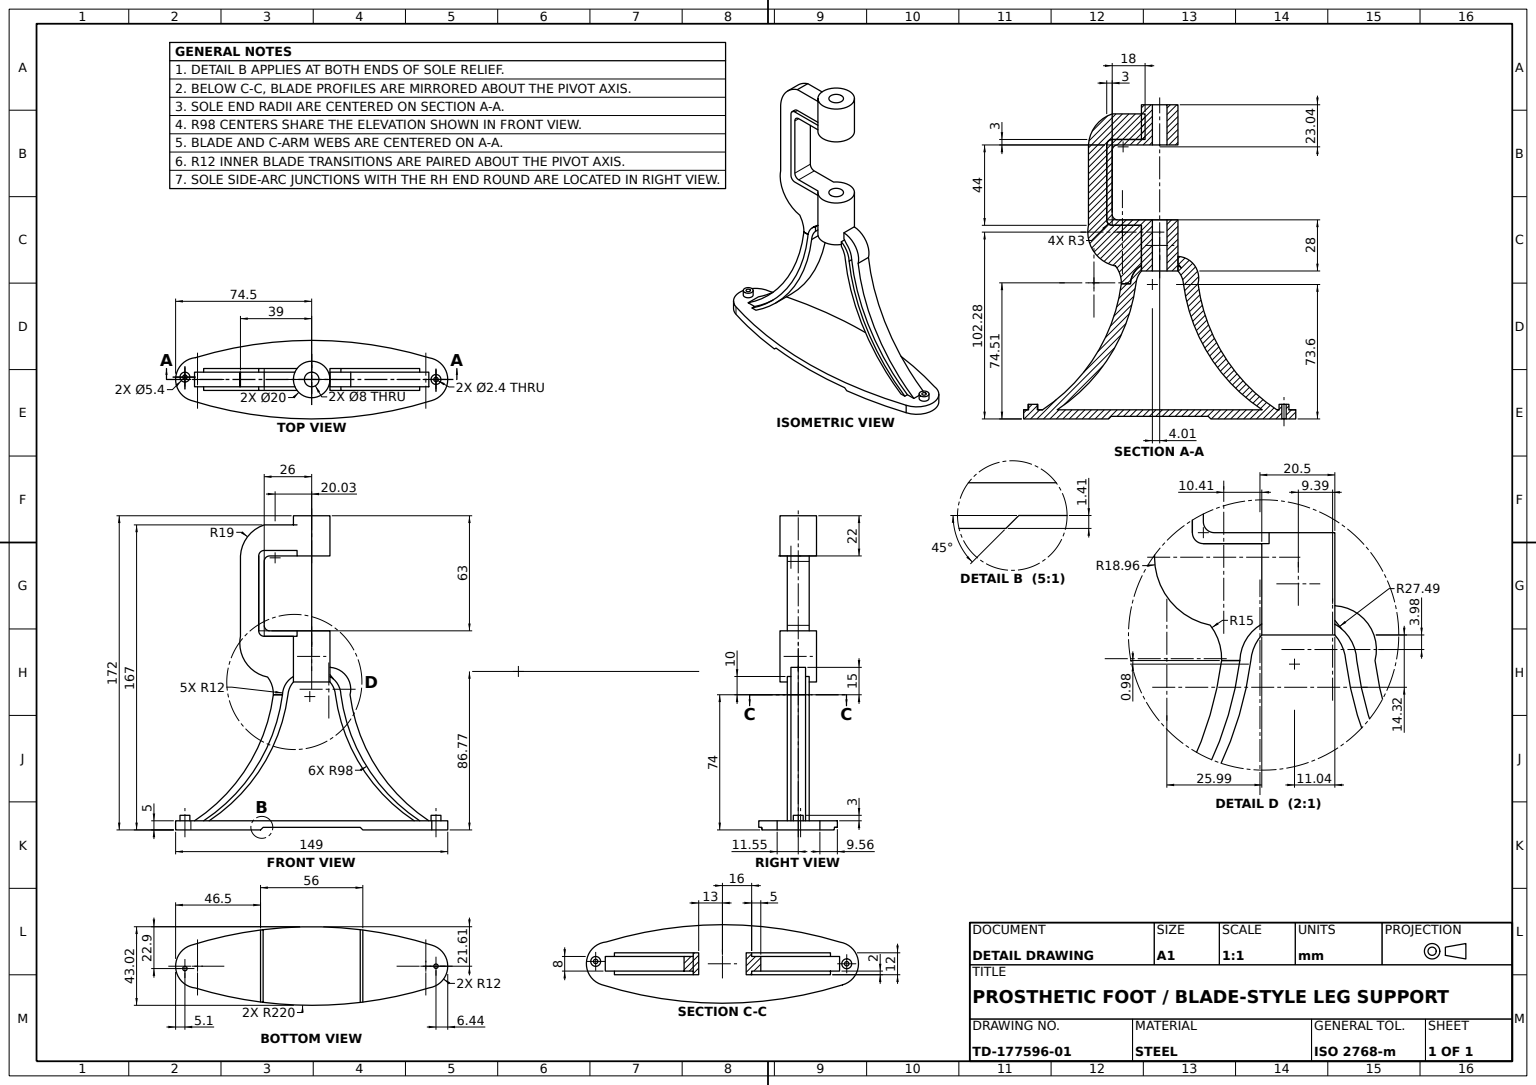
from build123d import *

# Parameters (mm, degrees)
BASE_PLATE_DEPTH             = 5
UPPER_PIVOT_BOSS_SKETCH_R    = 10
UPPER_PIVOT_BOSS_DEPTH       = 22
LOWER_PIVOT_BOSS_SKETCH_R    = 10
LOWER_PIVOT_BOSS_DEPTH       = 28
SUPPORT_LEGS_DEPTH           = 6
C_ARM_DEPTH                  = 6
LEG_RIBS_DEPTH               = 4
C_ARM_RIB_DEPTH              = 4
PIVOT_BORE_SKETCH_R          = 4
PIVOT_BORE_DEPTH             = 128
BASE_SCREW_BOSSES_SKETCH_R   = 2.697739099
BASE_SCREW_BOSSES_SKETCH_R_2 = 2.7
BASE_SCREW_BOSSES_DEPTH      = 3
BASE_SCREW_HOLES_SKETCH_R    = 1.2
BASE_SCREW_HOLES_DEPTH       = 33
PROFILE_TRIM_CUT_DEPTH       = 59


with BuildPart() as part:
    # Base Plate Sketch → Base Plate (new body)
    with BuildSketch(Plane(origin=(0, 0, 0), x_dir=(1, 0, 0), z_dir=(0, 1, 0))):
        with BuildLine():
            ThreePointArc((64.36610424, 11.854014297), (0.380988732, 21.413349806), (-63.618068043, 11.947799959))
            ThreePointArc((-63.618068043, 11.947799959), (-74.430459123, 1.290017486), (-66.146151353, -11.432654124))
            ThreePointArc((-66.146151353, -11.432654124), (-66.105249037, -11.445618349), (-66.064300627, -11.458436239))
            ThreePointArc((-66.064300627, -11.458436239), (-0.16489578, -21.609157542), (65.7488293, -11.551844363))
            ThreePointArc((65.7488293, -11.551844363), (74.479114791, 0.707678469), (64.36610424, 11.854014297))
        make_face()
    extrude(amount=BASE_PLATE_DEPTH)

    # Support Legs Sketch → Support Legs (add, symmetric)
    with BuildSketch(Plane.XY):
        with BuildLine():
            Line((-56.146151353, 5), (-59.146151353, 5))
            ThreePointArc((-59.146151353, 5), (-30.072320043, 34.809728437), (-16, 74))
            ThreePointArc((-16, 74), (-14.296453431, 79.777872059), (-10, 84))
            Line((-10, 84), (-10, 81))
            ThreePointArc((-10, 81), (-12.070047611, 77.744306119), (-13, 74))
            ThreePointArc((-13, 74), (-27.072320043, 34.809728437), (-56.146151353, 5))
        make_face()
        with BuildLine():
            Line((56.146151353, 5), (59.146151353, 5))
            ThreePointArc((59.146151353, 5), (30.072320043, 34.809728437), (16, 74))
            ThreePointArc((16, 74), (14.296453431, 79.777872059), (10, 84))
            Line((10, 84), (10, 81))
            ThreePointArc((10, 81), (12.070047611, 77.744306119), (13, 74))
            ThreePointArc((13, 74), (27.072320043, 34.809728437), (56.146151353, 5))
        make_face()
    extrude(amount=SUPPORT_LEGS_DEPTH, both=True)

    # Leg Ribs Sketch → Leg Ribs (add, symmetric)
    with BuildSketch(Plane.XY):
        with BuildLine():
            ThreePointArc((-16, 74), (-30.072320043, 34.809728437), (-59.146151353, 5))
            Line((-59.146151353, 5), (-64.146151353, 5))
            ThreePointArc((-64.146151353, 5), (-35.072320043, 34.809728437), (-21, 74))
            Line((-21, 74), (-16, 74))
        make_face()
        with BuildLine():
            ThreePointArc((16, 74), (30.072320043, 34.809728437), (59.146151353, 5))
            Line((59.146151353, 5), (64.146151353, 5))
            ThreePointArc((64.146151353, 5), (35.072320043, 34.809728437), (21, 74))
            ThreePointArc((21, 74), (19.061991309, 84.11212696), (10, 89))
            Line((10, 89), (10, 85))
            ThreePointArc((10, 85), (13.635056418, 79.84639441), (16, 74))
        make_face()
    extrude(amount=LEG_RIBS_DEPTH, both=True)

    # Base Screw Bosses Sketch → Base Screw Bosses (add)
    with BuildSketch(Plane(origin=(0, 5, 0), x_dir=(1, 0, 0), z_dir=(0, 1, 0))):
        with Locations(Location((68.059525022, 0, 0), (0, 0, 270))):
            Circle(BASE_SCREW_BOSSES_SKETCH_R)
        with Locations(Location((-69.403797915, 1.290017486, 0), (0, 0, 270))):
            Circle(BASE_SCREW_BOSSES_SKETCH_R_2)
    extrude(amount=BASE_SCREW_BOSSES_DEPTH)

    # Base Screw Holes Sketch → Base Screw Holes (cut)
    with BuildSketch(Plane(origin=(0, 8, 0), x_dir=(1, 0, 0), z_dir=(0, 1, 0))):
        with Locations(Location((68.059525022, 0, 0), (0, 0, 270))):
            Circle(BASE_SCREW_HOLES_SKETCH_R)
        with Locations(Location((-69.403797915, 1.290017486, 0), (0, 0, 270))):
            Circle(BASE_SCREW_HOLES_SKETCH_R)
    extrude(amount=-BASE_SCREW_HOLES_DEPTH, mode=Mode.SUBTRACT)

    # Profile Trim Sketch → Profile Trim Cut (cut)
    with BuildSketch(Plane.XY.offset(22)):
        Polygon((0, 0), (28, 0), (26.585786438, 1.414213562), (-26.585786438, 1.414213562), (-28, 0), align=None)
    extrude(amount=-PROFILE_TRIM_CUT_DEPTH, mode=Mode.SUBTRACT)


with BuildPart() as body_2:
    # Upper Pivot Boss Sketch → Upper Pivot Boss (new body)
    with BuildSketch(Plane(origin=(0, 172, 0), x_dir=(1, 0, 0), z_dir=(0, 1, 0))):
        with Locations(Location((0, 0, 0), (0, 0, 270))):
            Circle(UPPER_PIVOT_BOSS_SKETCH_R)
    extrude(amount=-UPPER_PIVOT_BOSS_DEPTH)



with BuildPart() as body_3:
    # Lower Pivot Boss Sketch → Lower Pivot Boss (new body)
    with BuildSketch(Plane(origin=(0, 109, 0), x_dir=(1, 0, 0), z_dir=(0, 1, 0))):
        with Locations(Location((0, 0, 0), (0, 0, 270))):
            Circle(LOWER_PIVOT_BOSS_SKETCH_R)
    extrude(amount=-LOWER_PIVOT_BOSS_DEPTH)


with BuildPart() as body_2_1:
    add(body_2.part)

    add(body_3.part)  # C-Arm merges body 3
    # C-Arm Sketch → C-Arm (add, symmetric)
    with BuildSketch(Plane.XY):
        with BuildLine():
            Line((-10, 153), (-26, 153))
            ThreePointArc((-26, 153), (-28.121320344, 152.121320344), (-29, 150))
            Line((-29, 150), (-29, 109))
            ThreePointArc((-29, 109), (-28.121320344, 106.878679656), (-26, 106))
            Line((-26, 106), (-10, 106))
            Line((-10, 106), (-7.9510102, 106))
            Line((-7.9510102, 106), (-7.9510102, 109))
            Line((-7.9510102, 109), (-10, 109))
            Line((-10, 109), (-23, 109))
            ThreePointArc((-23, 109), (-25.121320344, 109.878679656), (-26, 112))
            Line((-26, 112), (-26, 147))
            ThreePointArc((-26, 147), (-25.121320344, 149.121320344), (-23, 150))
            Line((-23, 150), (-10, 150))
            Line((-10, 150), (-7.9510102, 150))
            Line((-7.9510102, 150), (-7.9510102, 153))
            Line((-7.9510102, 153), (-10, 153))
        make_face()
    extrude(amount=C_ARM_DEPTH, both=True)

    # Pivot Bore Sketch → Pivot Bore (cut)
    with BuildSketch(Plane(origin=(0, 172, 0), x_dir=(1, 0, 0), z_dir=(0, 1, 0))):
        with Locations(Location((0, 0, 0), (0, 0, 270))):
            Circle(PIVOT_BORE_SKETCH_R)
    extrude(amount=-PIVOT_BORE_DEPTH, mode=Mode.SUBTRACT)


with BuildPart() as body_3_2:
    # C-Arm Rib Sketch → C-Arm Rib (new, symmetric)
    with BuildSketch(Plane.XY):
        with BuildLine():
            Line((-39, 150), (-39, 106))
            ThreePointArc((-39, 106), (-36.18490968, 91.76692418), (-24.130035795, 83.693189205))
            ThreePointArc((-24.130035795, 83.693189205), (-21.717038282, 79.120416406), (-21, 74))
            Line((-21, 74), (-16, 74))
            ThreePointArc((-16, 74), (-14.296453431, 79.777872059), (-10, 84))
            Line((-10, 84), (-10, 106))
            Line((-10, 106), (-26, 106))
            ThreePointArc((-26, 106), (-28.121320344, 106.878679656), (-29, 109))
            Line((-29, 109), (-29, 150))
            ThreePointArc((-29, 150), (-28.121320344, 152.121320344), (-26, 153))
            Line((-26, 153), (-8, 153))
            Line((-8, 153), (-8, 167))
            Line((-8, 167), (-26, 167))
            ThreePointArc((-26, 167), (-35.121127871, 160.504391901), (-39, 150))
        make_face()
    extrude(amount=C_ARM_RIB_DEPTH, both=True)


solid = Compound([part.part, body_2_1.part, body_3_2.part])
